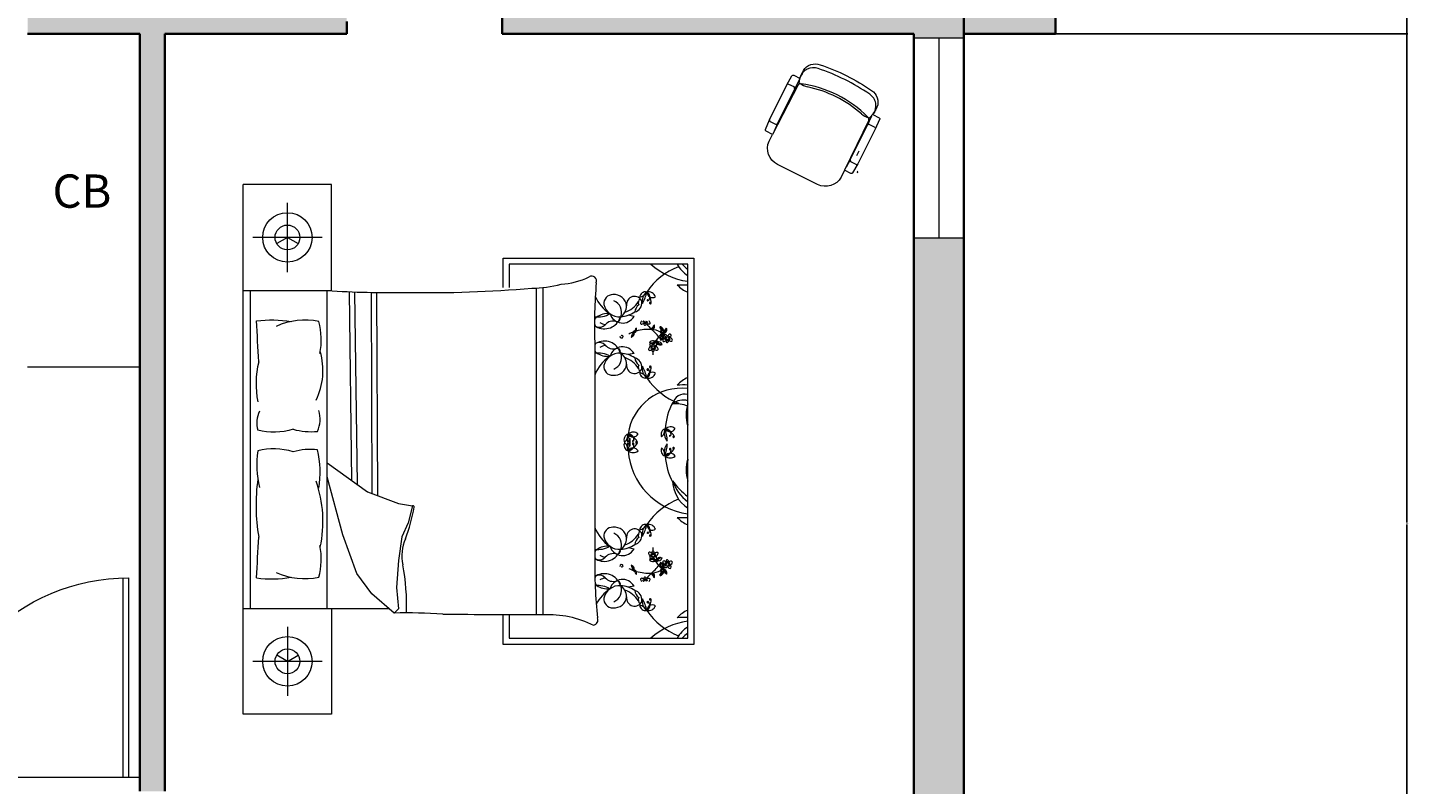
# Model space of a CAD drawing. Units: inches. Extents: x -36 to 442, y -676 to 151.
# Tile 7 of 8: x 193 to 442, y -134 to 2. Entities that reach past the tile are written whole.
import ezdxf

# ---------------------------------------------------------------- set-up
doc = ezdxf.new("R2010")
doc.units = ezdxf.units.IN
doc.header["$MEASUREMENT"] = 0
for name, color, linetype, lineweight in [('A-ANNO-DIMS', 2, 'Continuous', 18), ('A-ANNO-TEXT', 7, 'Continuous', 18), ('A-DOOR', 4, 'Continuous', 18), ('A-FLOR-CASE', 32, 'Continuous', 18), ('A-FURN', 9, 'Continuous', 13), ('A-GLAZ', 4, 'Continuous', 13), ('A-WALL', 7, 'Continuous', 35), ('A-WALL-PATT', 8, 'Continuous', 13)]:
    doc.layers.add(name, color=color, linetype=linetype, lineweight=lineweight)
doc.styles.get("Standard").update_dxf_attribs({"font": 'arial.ttf'})
doc.dimstyles.get("Standard").update_dxf_attribs({"dimtxt": 0.18, "dimasz": 0.18, "dimexe": 0.18, "dimexo": 0.0625, "dimgap": 0.09, "dimtad": 0, "dimtih": 1, "dimtoh": 1, "dimdec": 0, "dimzin": 0, "dimdsep": 46, "dimlunit": 3, "dimtxsty": 'Standard', "dimcen": 0.09, "dimadec": 0, "dimazin": 0, "dimtfac": 1, "dimtdec": 0, "dimtofl": 0, "dimtmove": 0, "dimatfit": 3, "dimfxl": 1, "dimtolj": 1, "dimtzin": 0, "dimarcsym": 0})

# ---------------------------------------------------------------- blocks, each defined once
blk = doc.blocks.new('DOOR-SWING-36IN')
for p, q in [((2, 0), (2, 36)), ((3, 0), (3, 36)), ((0, 0), (2, 0)), ((2, 0), (3, 0)), ((3, 0), (38, 0)), ((38, 0), (40, 0))]:
    blk.add_line(p, q)
blk.add_arc((2, 0), 36, 0, 90)
blk = doc.blocks.new('GLAZING-UNIT-36IN')
for p, q in [((0, 36), (0, 0)), ((4.5, 36), (4.5, 0)), ((9, 0), (9, 36))]:
    blk.add_line(p, q)
blk = doc.blocks.new('*D56')
at = {"layer": 'A-ANNO-DIMS', "color": 0, "lineweight": -2, "transparency": 16777216}
for p, q in [((378.8, 81.65), (442.22, 81.65)), ((442.04, 81.47), (442.04, 41.51)), ((442.04, 1.18), (442.04, 41.14)), ((378.8, 1), (442.22, 1))]:
    blk.add_line(p, q, dxfattribs=at)
at = {"layer": 'A-ANNO-DIMS', "color": 0, "transparency": 16777216}
for points in [[(442.01, 81.47), (442.07, 81.47), (442.04, 81.65)], [(442.01, 1.18), (442.07, 1.18), (442.04, 1)]]:
    blk.add_solid(points, dxfattribs=at)
at = {"layer": 'Defpoints', "color": 0, "transparency": 16777216}
for p in [(378.74, 81.65), (378.74, 1), (442.04, 1)]:
    blk.add_point(p, dxfattribs=at)
at = {"layer": 'A-ANNO-DIMS', "color": 0, "transparency": 16777216, "insert": (442.04, 41.32), "char_height": 0.18, "attachment_point": 5}
blk.add_mtext('\\A1;80.64', dxfattribs=at)
blk = doc.blocks.new('*D57')
at = {"layer": 'A-ANNO-DIMS', "color": 0, "lineweight": -2, "transparency": 16777216}
for p, q in [((378.8, 1), (442.22, 1)), ((442.04, 0.82), (442.04, -87.07)), ((442.04, -175.32), (442.04, -87.43)), ((387.8, -175.5), (442.22, -175.5))]:
    blk.add_line(p, q, dxfattribs=at)
at = {"layer": 'A-ANNO-DIMS', "color": 0, "transparency": 16777216}
for points in [[(442.01, 0.82), (442.07, 0.82), (442.04, 1)], [(442.01, -175.32), (442.07, -175.32), (442.04, -175.5)]]:
    blk.add_solid(points, dxfattribs=at)
at = {"layer": 'Defpoints', "color": 0, "transparency": 16777216}
for p in [(378.74, 1), (387.74, -175.5), (442.04, -175.5)]:
    blk.add_point(p, dxfattribs=at)
at = {"layer": 'A-ANNO-DIMS', "color": 0, "transparency": 16777216, "insert": (442.04, -87.25), "char_height": 0.18, "attachment_point": 5}
blk.add_mtext('\\A1;176.5', dxfattribs=at)

msp = doc.modelspace()

# ---------------------------------------------------------------- hatches: boundary and pattern name
at = {"layer": 'A-WALL-PATT'}
h = msp.add_hatch(color=256, dxfattribs=at)
h.dxf.hatch_style = 1
h.paths.add_polyline_path([(288, 113.503), (193.5, 113.503), (97.5, 113.503), (97.5, 104.864), (106.5, 104.864), (106.5, 104.503), (193.5, 104.503), (193.5, 5.503), (193.5, 1.003), (213.735, 1.003), (213.735, -135.497), (218.235, -135.497), (218.235, 1.003), (251, 1.003), (251, 3.253), (251, 5.503), (198, 5.503), (198, 104.503), (279, 104.503), (279, 104.209), (288, 104.209)])
h.paths.add_polyline_path([(378.735, 81.646), (362.235, 81.646), (288, 81.646), (288, 80.209), (279, 80.209), (279, 5.503), (279, 1.003), (353.235, 1.003), (353.235, 0.242), (362.235, 0.242), (362.235, 5.503), (288, 5.503), (288, 77.146), (362.235, 77.146), (374.235, 77.146), (374.235, 5.503), (362.235, 5.503), (362.235, 1.003), (374.235, 1.003), (378.735, 1.003), (378.735, 5.503), (378.735, 77.146)])
h.paths.add_polyline_path([(362.235, -35.758), (353.235, -35.758), (353.235, -196.997), (218.235, -196.997), (213.735, -196.997), (213.735, -205.997), (218.235, -205.997), (378.735, -205.997), (378.735, -205.779), (387.735, -205.779), (387.735, -202.472), (387.735, -196.997), (378.735, -196.997), (362.235, -196.997)])
h.paths.add_polyline_path([(218.235, -175.497), (215.985, -175.497), (213.735, -175.497), (213.735, -196.997), (218.235, -196.997)], flags=17)
h.paths.add_polyline_path([(158.235, -201.497), (98.235, -201.497), (98.235, -205.997), (158.235, -205.997)])
h.paths.add_polyline_path([(173.735, -130.997), (27.735, -130.997), (27.735, -35.267), (18.735, -35.267), (18.735, -138.68), (27.735, -138.68), (27.735, -135.497), (93.735, -135.497), (93.735, -201.497), (98.235, -201.497), (98.235, -135.497), (158.235, -135.497), (158.235, -173.497), (160.739, -173.497), (162.735, -173.497), (162.735, -135.497), (173.735, -135.497), (173.735, -133.017)])
h.paths.add_polyline_path([(98.235, -201.497), (93.735, -201.497), (93.735, -205.997), (98.235, -205.997)])
h.paths.add_polyline_path([(162.735, -201.497), (158.235, -201.497), (158.235, -205.997), (162.735, -205.997)])
h.paths.add_polyline_path([(63.735, -205.997), (63.735, -201.497), (27.735, -201.497), (27.735, -162.68), (18.735, -162.68), (18.735, -210.497), (63.735, -210.497)])
h.paths.add_polyline_path([(65.735, -203.604), (65.735, -201.497), (63.735, -201.497), (63.735, -205.997), (65.735, -205.997)])
h.paths.add_polyline_path([(165.5, 5.503), (106.5, 5.503), (106.5, 80.864), (97.5, 80.864), (97.5, 81.646), (6.735, 81.646), (2.235, 81.646), (2.235, 77.146), (2.235, 5.503), (2.235, 1.003), (6.735, 1.003), (18.735, 1.003), (18.735, 5.503), (6.735, 5.503), (6.735, 77.146), (97.5, 77.146), (97.5, 5.503), (18.735, 5.503), (18.735, 0.733), (27.735, 0.733), (27.735, 1.003), (165.5, 1.003), (165.5, 3.253)])
h.paths.add_polyline_path([(18.735, -201.497), (6.735, -201.497), (2.235, -201.497), (2.235, -210.497), (2.235, -354.497), (2.235, -363.497), (6.735, -363.497), (18.735, -363.497), (18.735, -358.997), (18.735, -354.497), (6.735, -354.497), (6.735, -210.497), (18.735, -210.497)])
h.paths.add_polyline_path([(63.735, -210.497), (54.735, -210.497), (54.735, -240.747), (63.735, -240.747)])
h.paths.add_polyline_path([(63.735, -336.747), (54.735, -336.747), (54.735, -354.497), (18.735, -354.497), (18.735, -358.997), (18.735, -363.497), (104.735, -363.497), (104.735, -361.247), (104.735, -358.997), (63.735, -358.997)])
h.paths.add_polyline_path([(27.735, -448.151), (18.735, -448.151), (18.735, -637.997), (72.735, -637.997), (72.735, -571.997), (183.235, -571.997), (183.235, -562.997), (57.197, -562.997), (51.735, -562.997), (51.735, -567.497), (57.197, -567.497), (63.735, -567.497), (63.735, -571.997), (63.735, -628.997), (27.735, -628.997), (27.735, -475.997), (27.735, -471.497)])
h.paths.add_polyline_path([(27.735, -363.497), (18.735, -363.497), (18.735, -412.151), (27.735, -412.151)])
h.paths.add_polyline_path([(161.235, -358.997), (132.735, -358.997), (132.735, -363.497), (156.735, -363.497), (156.735, -471.497), (51.735, -471.497), (51.735, -475.997), (63.735, -475.997), (63.735, -534.997), (65.985, -534.997), (68.235, -534.997), (68.235, -475.997), (161.235, -475.997)])
h.paths.add_polyline_path([(161.235, -511.997), (173.235, -511.997), (173.235, -502.997), (161.235, -502.997), (161.235, -475.997), (152.235, -475.997), (152.235, -534.997), (156.735, -534.997), (161.235, -534.997)], flags=17)
h.paths.add_polyline_path([(362.235, -502.997), (353.235, -502.997), (213.235, -502.997), (213.235, -507.497), (213.235, -511.997), (362.235, -511.997)])
h.paths.add_polyline_path([(242.235, -548.019), (233.235, -548.019), (233.235, -562.997), (223.235, -562.997), (223.235, -567.497), (223.235, -571.997), (242.235, -571.997)])
h.paths.add_polyline_path([(404.235, -502.997), (399.735, -502.997), (362.235, -502.997), (362.235, -511.997), (399.735, -511.997), (404.235, -511.997)])
h.paths.add_polyline_path([(362.235, -482.123), (353.235, -482.123), (353.235, -502.997), (362.235, -502.997)])
h.paths.add_polyline_path([(404.235, -295.997), (404.235, -286.997), (387.735, -286.997), (387.735, -295.997), (399.735, -295.997), (399.735, -502.997), (404.235, -502.997)])
h.paths.add_polyline_path([(362.235, -355.863), (353.235, -355.863), (353.235, -386.123), (362.235, -386.123)])
h.paths.add_polyline_path([(387.735, -286.997), (378.735, -286.997), (213.735, -286.997), (213.735, -295.997), (353.235, -295.997), (353.235, -295.863), (362.235, -295.863), (362.235, -295.997), (378.735, -295.997), (387.735, -295.997)])
h.paths.add_polyline_path([(387.735, -241.779), (378.735, -241.779), (378.735, -286.997), (387.735, -286.997)])
h.paths.add_polyline_path([(387.735, -175.497), (362.235, -175.497), (362.235, -184.497), (387.735, -184.497)], flags=17)
h.paths.add_polyline_path([(387.735, -184.497), (383.235, -184.497), (383.235, -192.497), (378.735, -192.497), (366.735, -192.497), (366.735, -184.497), (362.235, -184.497), (362.235, -196.997), (378.735, -196.997), (387.735, -196.997)], flags=17)
h.paths.add_polyline_path([(240.604, 40.967), (282.575, 40.967), (282.575, 63.356), (240.604, 63.356)], flags=25)

# ---------------------------------------------------------------- linework, layer by layer
at = {"layer": 'A-FLOR-CASE'}
msp.add_line((193.5, -58.997), (213.735, -58.997), dxfattribs=at)
at = {"layer": 'A-FURN', "ltscale": 0.03}
for p, q in [((331.738, -8.903), (332.638, -7.246)), ((332.564, -7.834), (332.752, -6.859)), ((332.912, -6.45), (333.341, -5.606)), ((332.353, -8.189), (327.751, -17.107)), ((328.615, -15.161), (331.738, -8.903)), ((331.627, -8.571), (330.686, -8.101)), ((327.342, -14.802), (328.283, -15.271)), ((345.085, -14.541), (340.727, -23.581)), ((344.885, -15.462), (345.667, -13.747)), ((345.241, -14.159), (345.906, -13.423)), ((328.615, -15.161), (328.042, -16.544)), ((341.763, -21.72), (344.885, -15.462)), ((345.217, -15.351), (346.158, -15.821)), ((341.763, -21.72), (341.002, -23.011)), ((342.815, -22.522), (341.874, -22.052)), ((342.955, -20.944), (343.372, -20.094))]:
    msp.add_line(p, q, dxfattribs=at)
at = {"layer": 'A-FURN'}
for p, q in [((232.366, -121.63), (232.366, -26.138)), ((240.323, -41.926), (240.323, -29.448)), ((246.562, -35.687), (234.084, -35.687)), ((279.176, -44.704), (279.176, -39.408)), ((279.176, -39.408), (313.575, -39.408)), ((313.575, -39.408), (313.575, -109.026)), ((280.283, -40.515), (280.283, -44.724)), ((312.469, -40.515), (280.283, -40.515)), ((312.469, -107.92), (312.469, -40.515)), ((286.323, -44.712), (286.323, -103.632)), ((233.591, -45.236), (233.591, -102.532)), ((247.456, -102.532), (247.456, -45.236)), ((251.423, -45.493), (251.9, -79.491)), ((252.403, -45.53), (252.893, -80.204)), ((255.41, -45.579), (255.554, -81.84)), ((256.39, -45.574), (256.54, -82.215)), ((285.132, -44.803), (285.132, -103.632)), ((302.788, -49.925), (301.709, -49.714)), ((295.703, -54.498), (295.703, -93.27)), ((302.788, -56.599), (301.709, -56.81)), ((247.456, -76.298), (254.74, -81.531)), ((250.294, -89.268), (247.456, -78.855)), ((254.74, -81.531), (260.346, -83.659)), ((260.346, -83.659), (262.858, -84.046)), ((262.858, -84.046), (262.085, -87.14)), ((252.807, -96.231), (250.294, -89.268)), ((262.085, -87.14), (260.925, -89.655)), ((260.925, -89.655), (260.346, -93.91)), ((302.788, -91.836), (301.709, -91.625)), ((260.346, -93.91), (259.959, -98.745)), ((255.513, -99.905), (252.807, -96.231)), ((259.959, -98.745), (260.346, -102.613)), ((302.788, -98.51), (301.709, -98.721)), ((259.572, -103.387), (255.513, -99.905)), ((232.366, -102.532), (258.576, -102.532)), ((260.346, -102.613), (259.572, -103.387)), ((279.176, -109.026), (279.176, -103.625)), ((280.283, -103.627), (280.283, -107.92)), ((240.323, -105.842), (240.323, -118.32)), ((313.575, -109.026), (279.176, -109.026)), ((280.283, -107.92), (312.469, -107.92)), ((246.562, -112.081), (234.084, -112.081))]:
    msp.add_line(p, q, dxfattribs=at)
at = {"layer": 'A-FURN', "ltscale": 0.03}
msp.add_lwpolyline([(346.555, -12.199), (346.346, -12.624, -0.029912), (346.004, -13.298, -0.0631929), (345.802, -13.538), (346.94, -14.106, -0.4142136), (347.051, -14.438), (346.269, -16.153), (343.147, -22.411), (343.147, -22.411), (343.147, -22.411), (342.19, -24.034, -0.4142136), (341.858, -24.145), (340.727, -23.581), (340.133, -24.814, -0.4039906), (335.846, -26.131), (328.649, -22.541, -0.4039906), (327.124, -18.323), (327.751, -17.107), (326.621, -16.543, -0.4142136), (326.51, -16.211), (327.231, -14.47), (330.354, -8.212), (331.254, -6.556, -0.4142136), (331.585, -6.445), (332.724, -7.013, -0.0631952), (332.794, -6.707, -0.029912), (333.126, -6.028), (333.341, -5.606, -0.1969574), (334.635, -4.542, -0.1563962), (336.313, -4.562, -0.0348091), (341.123, -6.547, -0.0348091), (345.602, -9.197, -0.1563962), (346.626, -10.525, -0.1969574)], format="xyb", close=True, dxfattribs=at)
at = {"layer": 'A-FURN'}
for points in [[(232.366, -45.236), (248.281, -45.236), (248.281, -26.138), (232.366, -26.138)], [(240.323, -35.687), (238.394, -36.801)], [(240.323, -35.687), (242.253, -36.801)], [(248.281, -102.532), (248.281, -121.63), (232.366, -121.63)], [(240.323, -112.081), (238.394, -110.967)], [(240.323, -112.081), (242.253, -110.967)]]:
    msp.add_lwpolyline(points, dxfattribs=at)
for points in [[(284.38, -44.829, 0.0561118), (289.634, -44.136, 0.0953413), (294.695, -42.794)], [(234.746, -50.721, -0.0748968), (240.983, -50.837, 0.4728166)], [(241.332, -70.254, -0.1409896), (234.969, -70.445, -0.2352448)], [(241.332, -74.332, 0.1409896), (234.969, -74.141, 0.2352448)], [(234.746, -97.047, 0.0748968), (240.983, -96.931, -0.4728166)], [(268.316, -103.587, 0.0012423), (286.435, -103.632, -0.1272016), (295.465, -105.547)]]:
    msp.add_lwpolyline(points, format="xyb", dxfattribs=at)
for centre, radius in [((240.323, -35.687), 4.456), ((240.323, -35.687), 2.228), ((308.811, -53.851), 0.243), ((306.248, -55.442), 0.243), ((306.248, -92.993), 0.243), ((308.811, -94.583), 0.243), ((240.323, -112.081), 4.456), ((240.323, -112.081), 2.228)]:
    msp.add_circle(centre, radius, dxfattribs=at)
at = {"layer": 'A-FURN', "ltscale": 0.03}
for centre, radius, start, end in [((335.102, -7.543), 2.447, 69.33312, 163.78228), ((324.476, -39.912), 36.513, 55.31099, 71.65919), ((330.575, -8.322), 0.247, 63.48361, 153.48361), ((331.516, -8.792), 0.247, 333.48361, 63.48361), ((332.732, -8.374), 0.422, 94.25862, 154.03485), ((332.828, -7.671), 0.309, 211.91025, 279.80308), ((335.198, -4.277), 4.446, 235.64869, 254.57345), ((329.876, -29.088), 21.326, 45.06486, 81.90236), ((329.876, -29.088), 20.939, 48.36888, 78.59834), ((343.948, -11.957), 2.447, 323.18495, 57.6341), ((327.453, -14.581), 0.247, 153.48361, 243.48361), ((346.5, -9.915), 4.446, 232.39378, 251.31854), ((345.214, -13.851), 0.309, 207.16414, 275.05697), ((344.709, -14.349), 0.422, 332.93238, 32.70861), ((328.394, -15.05), 0.247, 243.48361, 333.48361), ((345.106, -15.573), 0.247, 63.48361, 153.48361), ((341.984, -21.831), 0.247, 153.48361, 243.48361), ((342.925, -22.3), 0.247, 243.48361, 333.48361), ((342.864, -23.937), 0.247, 333.48361, 63.48361)]:
    msp.add_arc(centre, radius, start, end, dxfattribs=at)
at = {"layer": 'A-FURN'}
for centre, radius, start, end in [((315.382, -52.565), 12.47, 111.40921, 145.61345), ((314.149, -31.231), 12.47, 228.1144, 262.25504), ((315.819, -37.487), 6.076, 209.88843, 236.53828), ((316.952, -35.301), 7.572, 223.51858, 233.69643), ((295.179, -43.517), 0.87, 336.52186, 123.82642), ((388.579, -51.574), 92.922, 175.24024, 181.80351), ((314.414, -40.89), 5.07, 221.04544, 247.44526), ((311.689, -27.002), 17.253, 266.34809, 272.59189), ((259.127, 125.95), 171.584, 266.09997, 270.92818), ((265.365, 178.185), 223.823, 269.11454, 274.87351), ((302.428, -43.395), 7.227, 203.64533, 236.33288), ((298.958, -47.605), 1.612, 88.94622, 185.51443), ((299.188, -48.266), 2.282, 7.11425, 95.05515), ((298.323, -49.163), 2.216, 338.57785, 68.41813), ((299.711, -44.9), 4.508, 288.2955, 328.73863), ((302.865, -47.741), 1.433, 19.13116, 189.73602), ((302.434, -47.397), 1.79, 285.6955, 4.03098), ((304.418, -47.446), 0.878, 126.73195, 206.02445), ((304.846, -46.527), 1.034, 76.27204, 177.04841), ((303.273, -44.414), 2.13, 284.70312, 328.61733), ((306.244, -47.122), 1.971, 125.76571, 194.53465), ((296.575, -43.632), 8.724, 332.81761, 347.48274), ((305.386, -46.874), 1.383, 20.96132, 102.28847), ((306.132, -45.492), 1.041, 181.71311, 301.53669), ((302.717, -47.598), 3.154, 2.0648, 41.15983), ((304.618, -46.426), 1.02, 316.22381, 62.3173), ((305.205, -47.024), 0.0813, 20.26671, 316.22708), ((296.41, -46.045), 3.956, 259.24899, 301.17822), ((298.127, -53.081), 3.683, 85.26963, 124.21495), ((300.15, -47.11), 2.872, 193.079, 274.70666), ((300.73, -48.741), 2.374, 196.8663, 330.09146), ((298.681, -47.869), 2.774, 305.95986, 357.6409), ((300.074, -44.857), 5.124, 273.4924, 303.71172), ((304.813, -49.325), 1.906, 128.41745, 173.8338), ((305.714, -47.49), 0.155, 168.5166, 2.0648), ((305.636, -47.474), 0.0752, 52.05911, 168.5166), ((-674.028, -103.356), 910.296, 2.850225, 3.314791), ((243.487, -62.887), 12.308, 78.24166, 114.8684), ((233.628, -54.128), 12.797, 348.96311, 14.89607), ((296.76, -50.946), 1.15, 196.63434, 225.54831), ((296.76, -50.946), 1.15, 127.67503, 162.58143), ((297.438, -49.11), 3.043, 240.8249, 340.71782), ((296.532, -50.46), 1.429, 246.16459, 318.43469), ((297.988, -48.65), 2.745, 240.08513, 262.56401), ((299.065, -52.707), 1.958, 74.85287, 138.43469), ((299.732, -50.245), 0.593, 254.85287, 12.69594), ((298.127, -53.081), 3.683, 53.65552, 57.29887), ((303.476, -52.482), 0.501, 115.53786, 168.67439), ((301.774, -51.76), 1.509, 329.34401, 349.74122), ((305.437, -60.155), 7.909, 86.17232, 106.41582), ((300.568, -52.108), 2.693, 352.86976, 1.67361), ((304.137, -51.136), 0.188, 125.0752, 284.76444), ((304.426, -51.064), 0.406, 127.3642, 168.43627), ((304.108, -50.738), 0.585, 277.49685, 341.27373), ((304.572, -51.011), 0.232, 88.13253, 178.89195), ((305.04, -51.258), 0.503, 136.34618, 189.6513), ((304.751, -51.307), 0.21, 189.6513, 312.32085), ((304.803, -50.728), 0.243, 183.27684, 356.72316), ((305.562, -51.162), 0.796, 164.28291, 186.91484), ((304.624, -51.168), 0.398, 312.32085, 40.21108), ((305.466, -50.719), 0.565, 201.63824, 274.94696), ((304.718, -51.492), 0.738, 42.38963, 66.57243), ((312.167, -45.649), 9.067, 217.9541, 226.84587), ((305.253, -51.059), 0.401, 10.95974, 52.23791), ((305.499, -51.096), 0.187, 274.94696, 37.52629), ((306.126, -52.154), 0.195, 112.55835, 214.23425), ((306, -51.807), 0.458, 265.71315, 351.65678), ((305.598, -51.553), 0.8, 297.36586, 329.34401), ((304.992, -50.865), 1.534, 313.69288, 321.78988), ((306.689, -51.913), 0.501, 115.53786, 168.67439), ((304.988, -51.192), 1.509, 329.34401, 349.74122), ((303.781, -51.539), 2.693, 352.86976, 1.67361), ((307.568, -52.082), 0.272, 33.09787, 123.13641), ((301.587, -55.91), 7.105, 31.11559, 34.8118), ((307.175, -52.548), 0.735, 2.31716, 70.52013), ((307.429, -52.384), 0.281, 315.73542, 31.11559), ((307.453, -52.466), 0.633, 352.60083, 57.18452), ((307.876, -52.098), 0.735, 291.70871, 3.02993), ((302.63, -48.223), 7.105, 323.62539, 327.3216), ((308.457, -52.283), 0.272, 325.60767, 55.6462), ((297.438, -57.415), 3.043, 19.28218, 119.1751), ((296.532, -56.065), 1.429, 41.56531, 113.83541), ((300.518, -53.515), 0.299, 169.58644, 349.56155), ((300.631, -53.536), 0.184, 349.56155, 167.29493), ((305.437, -60.155), 7.909, 110.10592, 116.9968), ((302.784, -53.636), 0.501, 129.50559, 182.64212), ((301.345, -52.477), 1.509, 308.43876, 328.83597), ((301.082, -51.249), 2.693, 296.50636, 305.31021), ((301.06, -52.635), 1.534, 336.39009, 344.48709), ((302.732, -53.026), 0.195, 83.94573, 185.62162), ((301.952, -52.844), 0.8, 328.83597, 0.81412), ((302.366, -53.079), 0.458, 306.52319, 32.46683), ((302.913, -52.723), 0.195, 112.55835, 214.23425), ((302.786, -52.376), 0.458, 265.71315, 351.65678), ((302.384, -52.122), 0.8, 297.36586, 329.34401), ((301.779, -51.434), 1.534, 313.69288, 321.78988), ((305.886, -53.58), 1.109, 253.63009, 325.46314), ((306.198, -55.119), 0.784, 82.07481, 142.68955), ((306.109, -54.042), 0.805, 228.34199, 274.98936), ((305.637, -56.215), 3.965, 60.79592, 85.24398), ((297.194, -61.923), 13.048, 37.82556, 47.75876), ((306.134, -54.172), 0.674, 273.87739, 357.15012), ((306.983, -55.377), 0.767, 121.9501, 165.24419), ((306.396, -53.696), 0.652, 262.07481, 308.23927), ((310.903, -56.623), 4.756, 156.15226, 156.94993), ((306.704, -54.931), 0.241, 44.37319, 121.9501), ((307.448, -54.365), 0.674, 181.4625, 249.4747), ((307.333, -53.834), 0.652, 215.11283, 261.27729), ((307.855, -53.868), 1.109, 197.88895, 269.722), ((310.903, -56.623), 4.756, 130.18202, 149.45598), ((307.115, -55.254), 0.784, 20.66254, 81.27729), ((308.284, -53.914), 0.784, 139.38119, 199.99593), ((306.821, -53.345), 1.109, 310.93647, 22.76952), ((307.33, -53.407), 0.805, 285.64837, 332.29574), ((307.782, -52.729), 0.212, 135.73542, 318.12966), ((307.194, -52.979), 0.652, 319.38119, 5.54564), ((307.941, -52.728), 0.212, 68.24522, 250.63946), ((309.714, -56.716), 4.236, 111.70871, 116.21806), ((305.637, -56.215), 3.965, 47.50829, 55.99666), ((308.058, -52.323), 0.633, 252.8042, 349.69432), ((307.453, -53.456), 0.674, 331.18377, 51.67918), ((308.145, -54.26), 0.188, 125.0752, 284.76444), ((308.124, -52.269), 0.281, 248.24522, 323.62539), ((308.435, -54.188), 0.406, 93.63497, 168.43627), ((308.383, -53.546), 0.238, 138.29465, 276.24744), ((308.117, -53.862), 0.585, 277.49685, 341.27373), ((308.473, -53.583), 0.332, 358.57189, 143.89544), ((308.581, -54.135), 0.232, 88.13253, 178.89195), ((308.666, -53.322), 0.335, 208.84925, 269.93549), ((308.381, -53.401), 0.382, 274.21229, 318.15875), ((309.048, -54.382), 0.503, 136.34618, 189.6513), ((308.759, -54.431), 0.21, 189.6513, 312.32085), ((309.571, -54.286), 0.796, 164.28291, 186.91484), ((309.546, -53.786), 0.767, 121.9501, 165.24419), ((308.632, -54.291), 0.398, 312.32085, 40.21108), ((309.475, -53.843), 0.565, 201.63824, 274.94696), ((309.016, -53.491), 0.161, 262.86802, 7.09399), ((308.727, -54.616), 0.738, 42.38963, 66.57243), ((308.997, -53.356), 0.48, 278.56141, 22.59143), ((309.262, -54.183), 0.401, 10.95974, 118.78041), ((309.268, -53.34), 0.241, 44.37319, 121.9501), ((309.508, -54.22), 0.187, 274.94696, 37.52629), ((234.571, -59.651), 12.156, 333.87611, 16.17464), ((296.76, -55.579), 1.15, 134.45169, 156.71436), ((296.76, -55.579), 1.15, 203.28564, 232.32497), ((296.41, -60.479), 3.956, 58.82178, 100.28665), ((302.428, -63.13), 7.227, 123.66712, 158.50587), ((298.127, -53.443), 3.683, 235.78505, 274.73037), ((297.988, -57.874), 2.745, 97.43599, 119.91487), ((300.15, -59.414), 2.872, 85.29334, 166.921), ((299.065, -53.818), 1.958, 221.56531, 285.14713), ((300.73, -57.783), 2.374, 29.90854, 163.1337), ((298.323, -57.361), 2.216, 291.58187, 21.42215), ((299.732, -56.28), 0.593, 347.30406, 105.14713), ((298.127, -53.443), 3.683, 302.70113, 306.34448), ((298.681, -58.655), 2.774, 2.3591, 54.04014), ((300.074, -61.667), 5.124, 56.28828, 86.5076), ((305.582, -55.851), 0.188, 125.0752, 284.76444), ((305.871, -55.778), 0.406, 93.63497, 168.43627), ((305.82, -55.137), 0.238, 138.29465, 276.24744), ((305.553, -55.453), 0.585, 277.49685, 341.27373), ((305.91, -55.174), 0.332, 358.57189, 143.89544), ((306.018, -55.726), 0.232, 88.13253, 178.89195), ((306.103, -54.913), 0.335, 208.84925, 269.93549), ((305.817, -54.992), 0.382, 274.21229, 318.15875), ((306.485, -55.972), 0.503, 136.34618, 189.6513), ((306.196, -56.021), 0.21, 189.6513, 312.32085), ((310.903, -56.623), 4.756, 175.24147, 182.89291), ((307.007, -55.877), 0.796, 164.28291, 186.91484), ((306.069, -55.882), 0.398, 312.32085, 40.21108), ((306.912, -55.434), 0.565, 201.63824, 274.94696), ((306.453, -55.082), 0.161, 262.86802, 7.09399), ((306.163, -56.207), 0.738, 42.38963, 66.57243), ((306.433, -54.947), 0.48, 278.56141, 22.59143), ((306.698, -55.773), 0.401, 10.95974, 118.78041), ((306.944, -55.811), 0.187, 274.94696, 37.52629), ((307.509, -54.247), 0.805, 248.36273, 295.0101), ((251.455, -62.055), 16.787, 166.34271, 191.1841), ((298.958, -58.919), 1.612, 174.48557, 271.05378), ((299.188, -58.258), 2.282, 264.94485, 352.88575), ((299.711, -61.625), 4.508, 31.26137, 71.7045), ((302.865, -58.783), 1.433, 170.26398, 340.86884), ((304.813, -57.199), 1.906, 186.1662, 231.58255), ((302.434, -59.127), 1.79, 355.96902, 74.3045), ((304.418, -59.078), 0.878, 153.97555, 233.26805), ((306.244, -59.402), 1.971, 165.46535, 234.23429), ((296.575, -62.892), 8.724, 12.51726, 27.18239), ((302.717, -58.926), 3.154, 318.84017, 357.9352), ((304.618, -60.098), 1.02, 297.6827, 43.77619), ((305.257, -59.486), 0.135, 43.77619, 339.71835), ((305.714, -59.034), 0.155, 357.9352, 191.4834), ((305.636, -59.05), 0.0752, 191.4834, 307.94089), ((304.846, -59.997), 1.034, 182.95159, 283.72796), ((303.273, -62.111), 2.13, 31.38267, 75.29688), ((306.132, -61.033), 1.041, 58.46331, 178.28689), ((305.386, -59.65), 1.383, 257.71153, 339.03868), ((315.382, -53.959), 12.47, 214.38655, 248.59079), ((314.414, -65.634), 5.07, 112.55474, 138.95456), ((311.27, -72.513), 9.651, 82.86355, 171.81966), ((311.942, -66.143), 2.238, 76.38982, 169.07385), ((311.689, -79.523), 17.253, 87.40811, 93.65191), ((239.507, -69.135), 4.724, 153.34374, 196.10256), ((241.155, -68.496), 5.062, 335.01826, 18.54073), ((320.829, -71.155), 12.47, 152.5854, 175.53767), ((311.635, -67.826), 2.83, 72.86088, 131.90487), ((310.388, -71.265), 5.583, 68.11703, 96.61954), ((319.025, -67.668), 6.857, 162.9798, 196.45689), ((322.559, -70.384), 10.139, 174.36426, 175.62128), ((329.506, -75.725), 18.12, 160.09716, 160.27829), ((244.523, -58.997), 11.7, 254.17072, 275.98711), ((302.006, -72.132), 1.034, 106.19625, 206.97263), ((299.588, -71.085), 2.13, 314.62734, 358.54154), ((303.514, -71.951), 1.971, 155.68992, 224.45887), ((303.514, -73.3), 1.971, 135.54113, 204.31008), ((302.646, -72.164), 1.383, 50.88554, 132.21268), ((302.604, -70.593), 1.041, 211.63732, 331.4609), ((301.757, -72.159), 1.02, 346.14802, 92.24151), ((300.695, -74.123), 3.154, 31.98902, 71.08405), ((293.393, -73.749), 8.724, 2.74183, 17.40696), ((293.393, -71.502), 8.724, 342.59304, 357.25817), ((308.685, -71.178), 1.034, 106.19625, 206.97263), ((306.267, -70.131), 2.13, 314.62734, 358.54154), ((310.193, -70.996), 1.971, 155.68992, 224.45887), ((309.325, -71.209), 1.383, 50.88554, 132.21268), ((309.283, -69.639), 1.041, 211.63732, 331.4609), ((308.436, -71.204), 1.02, 346.14802, 92.24151), ((307.374, -73.168), 3.154, 31.98902, 71.08405), ((300.072, -72.795), 8.724, 2.74183, 17.40696), ((309.244, -71.429), 0.0813, 50.19092, 346.02088), ((309.842, -71.605), 0.0752, 81.98332, 198.44082), ((309.917, -71.58), 0.155, 198.44082, 31.98902), ((251.798, -76.648), 17.016, 171.52493, 193.95996), ((244.523, -85.588), 11.7, 84.01289, 105.82928), ((229.378, -77.918), 16.84, 349.86169, 13.62376), ((302.006, -73.119), 1.034, 153.02737, 253.80375), ((299.588, -74.166), 2.13, 1.45846, 45.37266), ((300.695, -71.129), 3.154, 288.91595, 328.01098), ((301.757, -73.093), 1.02, 267.75849, 13.85198), ((302.604, -74.658), 1.041, 28.5391, 148.36268), ((302.646, -73.088), 1.383, 227.78732, 309.11446), ((314.149, -73.142), 12.47, 184.46233, 262.25504), ((302.617, -72.881), 0.135, 13.85198, 309.92454), ((302.565, -72.384), 0.0813, 50.19092, 346.02088), ((303.163, -72.56), 0.0752, 81.98332, 198.44082), ((303.163, -72.692), 0.0752, 161.55918, 278.01668), ((303.238, -72.534), 0.155, 198.44082, 31.98902), ((303.238, -72.717), 0.155, 328.01098, 161.55918), ((308.685, -74.074), 1.034, 153.02737, 253.80375), ((306.267, -75.121), 2.13, 1.45846, 45.37266), ((310.193, -74.255), 1.971, 135.54113, 204.31008), ((300.072, -72.457), 8.724, 342.59304, 357.25817), ((307.374, -72.083), 3.154, 288.91595, 328.01098), ((308.436, -74.047), 1.02, 267.75849, 13.85198), ((309.283, -75.613), 1.041, 28.5391, 148.36268), ((309.296, -73.836), 0.135, 13.85198, 309.92454), ((309.842, -73.647), 0.0752, 161.55918, 278.01668), ((309.917, -73.672), 0.155, 328.01098, 161.55918), ((309.325, -74.043), 1.383, 227.78732, 309.11446), ((320.829, -74.097), 12.47, 184.46233, 207.4146), ((319.025, -77.584), 6.857, 163.54311, 197.0202), ((322.559, -74.867), 10.139, 184.37872, 185.63574), ((329.506, -69.527), 18.12, 199.72171, 199.90284), ((269.3, -83.963), 34.633, 172.21958, 189.49698), ((224.532, -86.904), 22.196, 348.03974, 19.26152), ((315.819, -79.398), 6.076, 181.27197, 236.53828), ((319.081, -73.232), 11.264, 214.01234, 234.05304), ((316.952, -77.211), 7.572, 197.85038, 233.69643), ((226.773, -77.416), 37.033, 340.11942, 349.33829), ((262.936, -84.262), 0.23, 358.86235, 109.75363), ((315.382, -94.476), 12.47, 111.40921, 145.61345), ((311.689, -68.912), 17.253, 266.34809, 272.59189), ((314.414, -82.801), 5.07, 221.04544, 247.44526), ((302.428, -85.305), 7.227, 201.49413, 236.33288), ((298.958, -89.515), 1.612, 88.94622, 185.51443), ((299.188, -90.176), 2.282, 7.11425, 95.05515), ((298.323, -91.073), 2.216, 338.57785, 68.41813), ((299.711, -86.81), 4.508, 288.2955, 328.73863), ((302.865, -89.652), 1.433, 19.13116, 189.73602), ((302.434, -89.308), 1.79, 285.6955, 4.03098), ((304.418, -89.357), 0.878, 126.73195, 206.02445), ((304.846, -88.437), 1.034, 76.27204, 177.04841), ((303.273, -86.324), 2.13, 284.70312, 328.61733), ((306.244, -89.033), 1.971, 125.76571, 194.53465), ((296.575, -85.543), 8.724, 332.81761, 347.48274), ((305.386, -88.784), 1.383, 20.96132, 102.28847), ((304.618, -88.337), 1.02, 316.22381, 62.3173), ((302.717, -89.509), 3.154, 2.0648, 41.15983), ((306.132, -87.402), 1.041, 181.71311, 301.53669), ((305.205, -88.934), 0.0813, 20.26671, 316.22708), ((305.714, -89.401), 0.155, 168.5166, 2.0648), ((305.636, -89.385), 0.0752, 52.05911, 168.5166), ((-674.028, -44.412), 910.296, 356.685209, 357.149775), ((233.628, -93.641), 12.797, 345.10393, 11.03689), ((268.714, -93.138), 7.773, 156.26158, 191.3392), ((296.41, -87.956), 3.956, 259.71335, 301.17822), ((296.76, -92.856), 1.15, 127.67503, 156.71436), ((297.438, -91.02), 3.043, 240.8249, 340.71782), ((298.127, -94.991), 3.683, 85.26963, 124.21495), ((300.15, -89.02), 2.872, 193.079, 274.70666), ((300.73, -90.652), 2.374, 196.8663, 330.09146), ((299.732, -92.155), 0.593, 254.85287, 12.69594), ((298.127, -94.991), 3.683, 53.65552, 57.29887), ((298.681, -89.78), 2.774, 305.95986, 357.6409), ((300.074, -86.768), 5.124, 273.4924, 303.71172), ((304.813, -91.235), 1.906, 128.41745, 173.8338), ((310.903, -91.812), 4.756, 177.10709, 184.75853), ((395.105, -94.409), 99.409, 179.34325, 185.68869), ((296.76, -92.856), 1.15, 203.22901, 225.54831), ((296.532, -92.37), 1.429, 246.16459, 318.43469), ((297.988, -90.561), 2.745, 240.08513, 262.56401), ((299.065, -94.617), 1.958, 74.85287, 138.43469), ((305.582, -92.584), 0.188, 75.23556, 234.9248), ((305.871, -92.656), 0.406, 191.56373, 266.36503), ((306.109, -94.393), 0.805, 85.01064, 131.65801), ((305.886, -94.854), 1.109, 34.53686, 106.36991), ((306.198, -93.315), 0.784, 217.31045, 277.92519), ((305.82, -93.298), 0.238, 83.75256, 221.70535), ((305.553, -92.982), 0.585, 18.72627, 82.50315), ((305.91, -93.261), 0.332, 216.10456, 1.42811), ((306.018, -92.709), 0.232, 181.10805, 271.86747), ((306.103, -93.522), 0.335, 90.06451, 151.15075), ((305.817, -93.443), 0.382, 41.84125, 85.78771), ((297.194, -86.511), 13.048, 312.24124, 322.17444), ((306.485, -92.463), 0.503, 170.3487, 223.65382), ((306.196, -92.413), 0.21, 47.67915, 170.3487), ((306.134, -94.262), 0.674, 2.84988, 86.12261), ((307.007, -92.558), 0.796, 173.08516, 195.71709), ((306.983, -93.058), 0.767, 194.75581, 238.0499), ((306.396, -94.738), 0.652, 51.76073, 97.92519), ((306.069, -92.553), 0.398, 319.78892, 47.67915), ((306.912, -93.001), 0.565, 85.05304, 158.36176), ((306.453, -93.353), 0.161, 352.90601, 97.13198), ((306.163, -92.228), 0.738, 293.42757, 317.61037), ((306.698, -92.661), 0.401, 241.21959, 349.04026), ((306.433, -93.488), 0.48, 337.40857, 81.43859), ((310.903, -91.812), 4.756, 203.05007, 203.84774), ((306.704, -93.504), 0.241, 238.0499, 315.62681), ((307.448, -94.07), 0.674, 110.5253, 178.5375), ((307.855, -94.566), 1.109, 90.278, 162.11105), ((307.333, -94.601), 0.652, 98.72271, 144.88717), ((310.903, -91.812), 4.756, 210.54402, 229.81798), ((306.944, -92.624), 0.187, 322.47371, 85.05304), ((307.509, -94.188), 0.805, 64.9899, 111.63727), ((307.115, -93.181), 0.784, 278.72271, 339.33746), ((308.284, -94.521), 0.784, 160.00407, 220.61881), ((306.821, -95.09), 1.109, 337.23048, 49.06353), ((307.33, -95.028), 0.805, 27.70426, 74.35163), ((308.145, -94.175), 0.188, 75.23556, 234.9248), ((308.435, -94.247), 0.406, 191.56373, 266.36503), ((308.117, -94.573), 0.585, 18.72627, 82.50315), ((308.581, -94.3), 0.232, 181.10805, 271.86747), ((309.048, -94.053), 0.503, 170.3487, 223.65382), ((308.759, -94.004), 0.21, 47.67915, 170.3487), ((309.571, -94.149), 0.796, 173.08516, 195.71709), ((308.632, -94.143), 0.398, 319.78892, 47.67915), ((309.475, -94.592), 0.565, 85.05304, 158.36176), ((308.727, -93.819), 0.738, 293.42757, 317.61037), ((309.262, -94.252), 0.401, 241.21959, 349.04026), ((309.508, -94.215), 0.187, 322.47371, 85.05304), ((243.487, -84.881), 12.308, 245.1316, 281.75834), ((225.756, -101.753), 36.04, 357.45188, 11.3392), ((296.76, -97.489), 1.15, 134.45169, 153.55801), ((297.438, -99.325), 3.043, 19.28218, 119.1751), ((296.532, -97.975), 1.429, 41.56531, 113.83541), ((299.065, -95.728), 1.958, 221.56531, 285.14713), ((300.518, -94.919), 0.299, 10.43845, 190.41356), ((300.631, -94.899), 0.184, 192.70507, 10.43845), ((305.437, -88.28), 7.909, 243.0032, 249.89408), ((302.784, -94.799), 0.501, 177.35788, 230.49441), ((301.345, -95.958), 1.509, 31.16403, 51.56124), ((301.082, -97.185), 2.693, 54.68979, 63.49364), ((301.06, -95.8), 1.534, 15.51291, 23.60991), ((302.732, -95.409), 0.195, 174.37838, 276.05427), ((301.952, -95.591), 0.8, 359.18588, 31.16403), ((302.366, -95.356), 0.458, 327.53317, 53.47681), ((302.913, -95.712), 0.195, 145.76575, 247.44165), ((302.786, -96.059), 0.458, 8.34322, 94.28685), ((302.384, -96.313), 0.8, 30.65599, 62.63414), ((301.779, -97.001), 1.534, 38.21012, 46.30712), ((303.476, -95.953), 0.501, 191.32561, 244.46214), ((301.774, -96.674), 1.509, 10.25878, 30.65599), ((305.437, -88.28), 7.909, 253.58418, 273.82768), ((300.568, -96.327), 2.693, 358.32639, 7.13024), ((304.751, -97.128), 0.21, 47.67915, 170.3487), ((304.624, -97.267), 0.398, 319.78892, 47.67915), ((312.167, -102.785), 9.067, 133.15413, 142.0459), ((306.126, -96.28), 0.195, 145.76575, 247.44165), ((305.637, -92.22), 3.965, 274.75602, 299.20408), ((306, -96.628), 0.458, 8.34322, 94.28685), ((305.598, -96.882), 0.8, 30.65599, 62.63414), ((304.992, -97.57), 1.534, 38.21012, 46.30712), ((306.689, -96.522), 0.501, 191.32561, 244.46214), ((304.988, -97.243), 1.509, 10.25878, 30.65599), ((303.781, -96.896), 2.693, 358.32639, 7.13024), ((307.175, -95.887), 0.735, 289.47987, 357.68284), ((301.587, -92.524), 7.105, 325.1882, 328.88441), ((307.568, -96.353), 0.272, 236.86359, 326.90213), ((307.782, -95.706), 0.212, 41.87034, 224.26458), ((307.429, -96.05), 0.281, 328.88441, 44.26458), ((307.194, -95.456), 0.652, 354.45436, 40.61881), ((307.941, -95.707), 0.212, 109.36054, 291.75478), ((307.453, -95.969), 0.633, 302.81548, 7.39917), ((309.714, -91.719), 4.236, 243.78194, 248.29129), ((305.637, -92.22), 3.965, 304.00334, 312.49171), ((307.453, -94.978), 0.674, 308.32082, 28.81623), ((308.058, -96.112), 0.633, 10.30568, 107.1958), ((308.124, -96.165), 0.281, 36.37461, 111.75478), ((308.383, -94.889), 0.238, 83.75256, 221.70535), ((307.876, -96.337), 0.735, 356.97007, 68.29129), ((308.473, -94.852), 0.332, 216.10456, 1.42811), ((302.63, -100.212), 7.105, 32.6784, 36.37461), ((308.666, -95.113), 0.335, 90.06451, 151.15075), ((308.381, -95.033), 0.382, 41.84125, 85.78771), ((308.457, -96.152), 0.272, 304.3538, 34.39233), ((309.546, -94.648), 0.767, 194.75581, 238.0499), ((309.016, -94.943), 0.161, 352.90601, 97.13198), ((308.997, -95.079), 0.48, 337.40857, 81.43859), ((309.268, -95.094), 0.241, 238.0499, 315.62681), ((296.76, -97.489), 1.15, 210.0293, 232.32497), ((296.41, -102.389), 3.956, 58.82178, 99.15542), ((302.428, -105.04), 7.227, 123.66712, 153.29966), ((298.127, -95.354), 3.683, 235.78505, 274.73037), ((297.988, -99.785), 2.745, 97.43599, 119.91487), ((300.15, -101.325), 2.872, 85.29334, 166.921), ((300.73, -99.693), 2.374, 29.90854, 163.1337), ((298.323, -99.272), 2.216, 291.58187, 21.42215), ((299.732, -98.19), 0.593, 347.30406, 105.14713), ((298.127, -95.354), 3.683, 302.70113, 306.34448), ((298.681, -100.566), 2.774, 2.3591, 54.04014), ((300.074, -103.577), 5.124, 56.28828, 86.5076), ((299.711, -103.535), 4.508, 31.26137, 71.7045), ((302.434, -101.038), 1.79, 355.96902, 74.3045), ((304.813, -99.11), 1.906, 186.1662, 231.58255), ((304.137, -97.298), 0.188, 75.23556, 234.9248), ((304.426, -97.371), 0.406, 191.56373, 232.6358), ((304.108, -97.696), 0.585, 18.72627, 82.50315), ((304.572, -97.424), 0.232, 181.10805, 271.86747), ((305.04, -97.177), 0.503, 170.3487, 223.65382), ((304.803, -97.707), 0.243, 3.27684, 176.72316), ((305.562, -97.272), 0.796, 173.08516, 195.71709), ((305.466, -97.716), 0.565, 85.05304, 158.36176), ((304.718, -96.942), 0.738, 293.42757, 317.61037), ((305.253, -97.376), 0.401, 307.76209, 349.04026), ((305.499, -97.338), 0.187, 322.47371, 85.05304), ((298.958, -100.83), 1.612, 174.48557, 271.05378), ((299.188, -100.169), 2.282, 264.94485, 352.88575), ((302.865, -100.694), 1.433, 170.26398, 340.86884), ((304.418, -100.989), 0.878, 153.97555, 233.26805), ((303.273, -104.021), 2.13, 31.38267, 75.29688), ((304.846, -101.908), 1.034, 182.95159, 283.72796), ((306.244, -101.312), 1.971, 165.46535, 234.23429), ((296.575, -104.803), 8.724, 12.51726, 27.18239), ((302.717, -100.836), 3.154, 318.84017, 357.9352), ((304.618, -102.009), 1.02, 297.6827, 43.77619), ((306.132, -102.943), 1.041, 58.46331, 178.28689), ((305.257, -101.396), 0.135, 43.77619, 339.71835), ((305.714, -100.944), 0.155, 357.9352, 191.4834), ((305.636, -100.96), 0.0752, 191.4834, 307.94089), ((261.946, -190.944), 87.589, 85.82941, 91.55305), ((295.404, -104.668), 0.881, 273.97998, 27.34124), ((305.386, -101.561), 1.383, 257.71153, 339.03868), ((315.382, -95.869), 12.47, 214.38655, 248.59079), ((314.414, -107.545), 5.07, 112.55474, 138.95456), ((311.689, -121.433), 17.253, 87.40811, 93.65191), ((314.149, -117.203), 12.47, 97.74496, 131.8856), ((315.819, -110.948), 6.076, 123.46172, 150.11157), ((316.952, -113.134), 7.572, 126.30357, 136.48142)]:
    msp.add_arc(centre, radius, start, end, dxfattribs=at)
at = {"layer": 'A-GLAZ'}
for p, q in [((362.235, 0.242), (353.235, 0.242)), ((353.235, -35.758), (362.235, -35.758))]:
    msp.add_line(p, q, dxfattribs=at)
at = {"layer": 'A-WALL'}
for p, q in [((279, 5.503), (279, 1.003)), ((362.235, 5.503), (362.235, -196.997)), ((378.735, 1.003), (378.735, 5.503)), ((251, 3.253), (251, 1.003)), ((193.5, 1.003), (213.735, 1.003)), ((213.735, 1.003), (213.735, -135.497)), ((218.235, 1.003), (218.235, -135.497)), ((218.235, 1.003), (251, 1.003)), ((279, 1.003), (353.235, 1.003)), ((353.235, 1.003), (353.235, -196.997)), ((362.235, 1.003), (374.235, 1.003)), ((374.235, 1.003), (378.735, 1.003))]:
    msp.add_line(p, q, dxfattribs=at)

# ---------------------------------------------------------------- block references
at = {"layer": 'A-DOOR', "extrusion": (0, 0, -1), "zscale": -1}
msp.add_blockref('DOOR-SWING-36IN', (-213.735, -133.017), dxfattribs=at)
at = {"layer": 'A-GLAZ'}
msp.add_blockref('GLAZING-UNIT-36IN', (353.235, -35.758), dxfattribs=at)

# ---------------------------------------------------------------- texts
at = {"layer": 'A-ANNO-TEXT', "insert": (197.99, -24.334), "char_height": 6, "attachment_point": 1}
msp.add_mtext('CB', dxfattribs=at)

# ---------------------------------------------------------------- dimensions: what is measured, and where the dimension line sits
at = {"layer": 'A-ANNO-DIMS'}
for base, p1, p2, override, picture, middle in [((442.035, 1.003), (378.735, 81.646), (378.735, 1.003), {"dimdec": 2, "dimlfac": 1, "dimrnd": 0, "dimzin": 0, "dimdsep": 46, "dimlunit": 2}, '*D56', (442.035, 41.324)), ((442.035, -175.497), (378.735, 1.003), (387.735, -175.497), {"dimdec": 1, "dimlfac": 1, "dimrnd": 0, "dimzin": 0, "dimdsep": 46, "dimlunit": 2}, '*D57', (442.035, -87.247))]:
    dim = msp.add_linear_dim(base=base, p1=p1, p2=p2, angle=90, dimstyle='Standard', override=override, dxfattribs=at)
    dim.commit()
    dim.dimension.update_dxf_attribs({"geometry": picture, "text_midpoint": middle})

doc.saveas('drawing.dxf')
